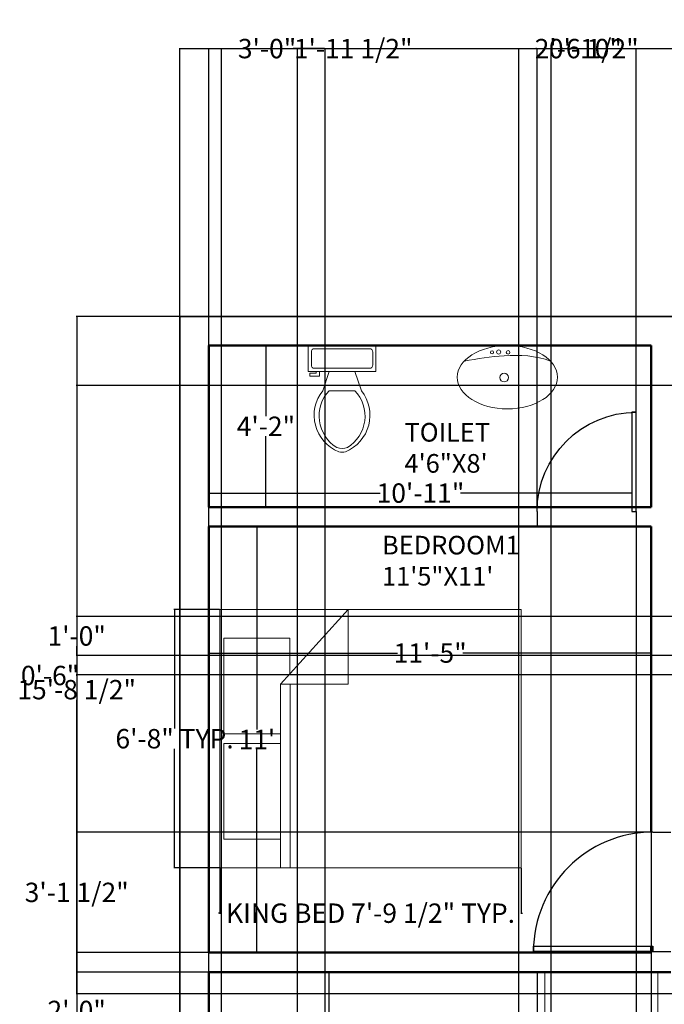
# Model space of a CAD drawing. Units: inches. Extents: x -56 to 545, y -536 to 185.
# Tile 5 of 7: x -56 to 144, y -120 to 185. Entities that reach past the tile are written whole.
import ezdxf

# ---------------------------------------------------------------- set-up
doc = ezdxf.new("R2010")
doc.units = ezdxf.units.IN
doc.header["$MEASUREMENT"] = 0
for name, color, linetype, lineweight in [('A-ANNO-DIMS', 2, 'Continuous', 18), ('A-AREA-IDEN', 4, 'Continuous', 25), ('A-DOOR', 4, 'Continuous', 25), ('A-EQPM', 9, 'Continuous', 18), ('A-FLOR-CASE', 8, 'Continuous', 25), ('A-FLOR-FIXT', 8, 'Continuous', 18), ('A-FURN', 8, 'Continuous', 18), ('A-WALL', 7, 'Continuous', 50), ('C-PROP', 7, 'Continuous', 35)]:
    doc.layers.add(name, color=color, linetype=linetype, lineweight=lineweight)
doc.styles.get("Standard").update_dxf_attribs({"font": 'arial.ttf'})
doc.dimstyles.get("Standard").update_dxf_attribs({"dimtxt": 6, "dimasz": 0.18, "dimexe": 0.18, "dimexo": 0.0625, "dimgap": 0.09, "dimtad": 0, "dimtih": 1, "dimtoh": 1, "dimdec": 0, "dimzin": 0, "dimdsep": 46, "dimlunit": 3, "dimtxsty": 'Standard', "dimcen": 0.09, "dimclrd": 3, "dimclre": 3, "dimclrt": 3, "dimadec": 0, "dimazin": 0, "dimtfac": 1, "dimtdec": 0, "dimtofl": 0, "dimtmove": 0, "dimatfit": 3, "dimfxl": 1, "dimtolj": 1, "dimtzin": 0, "dimarcsym": 0})

# ---------------------------------------------------------------- blocks, each defined once
blk = doc.blocks.new('CAMAKING')
for points in [[(0.8635, 0), (-0.8635, 0)], [(-0.8635, -2.0147), (-0.8635, 0)], [(0.8635, 0), (0.8635, -2.0147)], [(-0.6723, -0.4077), (-0.6723, -0.0281)], [(-0.6723, -0.0281), (-0.0328, -0.0281)], [(-0.0328, -0.0281), (-0.0328, -0.4077)], [(0.6716, -0.027), (0.0319, -0.027)], [(0.0319, -0.027), (0.0319, -0.4077)], [(0.6716, -0.4686), (0.6716, -0.027)], [(0.3645, -0.4056), (-0.8635, -0.4056)], [(0.8635, -0.857), (0.3645, -0.4056)], [(0.3645, -0.4702), (0.3645, -0.4056)], [(-0.8635, -0.4702), (0.3645, -0.4702)], [(0.3645, -0.4702), (0.3645, -0.857)], [(0.4362, -0.4686), (0.6716, -0.4686)], [(0.3645, -0.857), (0.8635, -0.857)], [(0.8635, -2.0147), (-0.8635, -2.0147)]]:
    blk.add_lwpolyline(points)
blk = doc.blocks.new('*U5')
for p, q in [((9.5, -6), (9.5, -2)), ((-10, -8.5), (-8, -8.5)), ((-10, -9.5), (-10, -8.5)), ((-8, -8.5), (-8, -8)), ((-7, -8), (-7, -9.5)), ((-4, -8), (-6, -14)), ((4, -8), (6, -14)), ((-7, -9.5), (-10, -9.5)), ((4, -14), (-4, -14))]:
    blk.add_line(p, q)
blk.add_lwpolyline([(10.5, -8), (10.5, 0), (-10.5, 0), (-10.5, -8)], close=True)
for points in [[(-9.5, -2), (-9.5, -6)], [(8.5, -1), (-8.5, -1)], [(-8.5, -7), (8.5, -7)]]:
    blk.add_lwpolyline(points)
for centre, radius, start, end in [((-8.62, -1.88), 0.884, 81.8699, 188.1301), ((8.62, -1.88), 0.884, 351.8699, 98.1301), ((-8.62, -6.12), 0.884, 171.8699, 278.1301), ((8.62, -6.12), 0.884, 261.8699, 8.1301), ((3.52, -21.58), 12.17, 141.4691, 247.9714), ((4.2, -21.82), 11.33, 136.3677, 238.9468), ((-3.52, -21.58), 12.17, 292.0284, 38.5307), ((-4.2, -21.82), 11.33, 301.053, 43.6321), ((0, -27.88), 4, 245.7318, 294.2682), ((0, -29), 4, 254.8605, 285.1395)]:
    blk.add_arc(centre, radius, start, end)
blk = doc.blocks.new('*U7')
for p, q in [((0, 0), (0, -6)), ((40, 0), (40, -6))]:
    blk.add_line(p, q)
blk.add_lwpolyline([(0, 0), (0, 40), (1.75, 40), (1.75, 0)], close=True)
blk.add_arc((0, 0), 40, 0, 90)
blk = doc.blocks.new('*D20')
at = {"layer": 'A-ANNO-DIMS', "color": 0, "lineweight": -2, "transparency": 16777216}
for p, q in [((96.89, -109.84), (40.02, -109.84)), ((40.2, -110.02), (40.2, -166.69)), ((40.2, -229.66), (40.2, -172.99)), ((96.89, -229.84), (40.02, -229.84))]:
    blk.add_line(p, q, dxfattribs=at)
at = {"layer": 'A-ANNO-DIMS', "color": 0, "transparency": 16777216}
for points in [[(40.17, -110.02), (40.23, -110.02), (40.2, -109.84)], [(40.17, -229.66), (40.23, -229.66), (40.2, -229.84)]]:
    blk.add_solid(points, dxfattribs=at)
at = {"layer": 'Defpoints', "color": 0, "transparency": 16777216}
for p in [(40.2, -109.84), (96.96, -109.84), (96.96, -229.84)]:
    blk.add_point(p, dxfattribs=at)
at = {"layer": 'A-ANNO-DIMS', "color": 0, "transparency": 16777216, "insert": (40.2, -169.84), "char_height": 6, "attachment_point": 5}
blk.add_mtext("\\A1;10'", dxfattribs=at)
blk = doc.blocks.new('*D22')
at = {"layer": 'A-ANNO-DIMS', "color": 0, "lineweight": -2, "transparency": 16777216}
for p, q in [((17.82, 28.16), (17.7, 28.16)), ((17.88, 27.98), (17.88, -34.74)), ((17.88, -103.66), (17.88, -40.94)), ((17.82, -103.84), (17.7, -103.84))]:
    blk.add_line(p, q, dxfattribs=at)
at = {"layer": 'A-ANNO-DIMS', "color": 0, "transparency": 16777216}
for points in [[(17.85, 27.98), (17.91, 27.98), (17.88, 28.16)], [(17.85, -103.66), (17.91, -103.66), (17.88, -103.84)]]:
    blk.add_solid(points, dxfattribs=at)
at = {"layer": 'Defpoints', "color": 0, "transparency": 16777216}
for p in [(17.88, 28.16), (17.88, 28.16), (17.88, -103.84)]:
    blk.add_point(p, dxfattribs=at)
at = {"layer": 'A-ANNO-DIMS', "color": 0, "transparency": 16777216, "insert": (17.88, -37.84), "char_height": 6, "attachment_point": 5}
blk.add_mtext("\\A1;11'", dxfattribs=at)
blk = doc.blocks.new('*D23')
at = {"layer": 'A-ANNO-DIMS', "color": 0, "lineweight": -2, "transparency": 16777216}
for p, q in [((3.03, 8), (3.03, -11.25)), ((140.03, 8), (140.03, -11.25)), ((3.21, -11.07), (61.42, -11.07)), ((139.85, -11.07), (81.65, -11.07))]:
    blk.add_line(p, q, dxfattribs=at)
at = {"layer": 'A-ANNO-DIMS', "color": 0, "transparency": 16777216}
for points in [[(3.21, -11.04), (3.21, -11.1), (3.03, -11.07)], [(139.85, -11.04), (139.85, -11.1), (140.03, -11.07)]]:
    blk.add_solid(points, dxfattribs=at)
at = {"layer": 'Defpoints', "color": 0, "transparency": 16777216}
for p in [(3.03, 8.06), (140.03, 8.06), (140.03, -11.07)]:
    blk.add_point(p, dxfattribs=at)
at = {"layer": 'A-ANNO-DIMS', "color": 0, "transparency": 16777216, "insert": (71.53, -11.07), "char_height": 6, "attachment_point": 5}
blk.add_mtext('\\A1;11\'-5"', dxfattribs=at)
blk = doc.blocks.new('*D24')
at = {"layer": 'A-ANNO-DIMS', "color": 0, "lineweight": -2, "transparency": 16777216}
for p, q in [((20.61, 84.16), (20.49, 84.16)), ((20.67, 83.98), (20.67, 62.26)), ((20.67, 34.34), (20.67, 56.06)), ((20.61, 34.16), (20.49, 34.16))]:
    blk.add_line(p, q, dxfattribs=at)
at = {"layer": 'A-ANNO-DIMS', "color": 0, "transparency": 16777216}
for points in [[(20.64, 83.98), (20.7, 83.98), (20.67, 84.16)], [(20.64, 34.34), (20.7, 34.34), (20.67, 34.16)]]:
    blk.add_solid(points, dxfattribs=at)
at = {"layer": 'Defpoints', "color": 0, "transparency": 16777216}
for p in [(20.67, 84.16), (20.67, 84.16), (20.67, 34.16)]:
    blk.add_point(p, dxfattribs=at)
at = {"layer": 'A-ANNO-DIMS', "color": 0, "transparency": 16777216, "insert": (20.67, 59.16), "char_height": 6, "attachment_point": 5}
blk.add_mtext('\\A1;4\'-2"', dxfattribs=at)
blk = doc.blocks.new('*D25')
at = {"layer": 'A-ANNO-DIMS', "color": 0, "lineweight": -2, "transparency": 16777216}
for p, q in [((3.03, 53.76), (3.03, 38.29)), ((134.04, 53.76), (134.04, 38.29)), ((3.21, 38.47), (56.09, 38.47)), ((133.86, 38.47), (80.98, 38.47))]:
    blk.add_line(p, q, dxfattribs=at)
at = {"layer": 'A-ANNO-DIMS', "color": 0, "transparency": 16777216}
for points in [[(3.21, 38.5), (3.21, 38.44), (3.03, 38.47)], [(133.86, 38.5), (133.86, 38.44), (134.04, 38.47)]]:
    blk.add_solid(points, dxfattribs=at)
at = {"layer": 'Defpoints', "color": 0, "transparency": 16777216}
for p in [(3.03, 53.82), (134.04, 53.82), (134.04, 38.47)]:
    blk.add_point(p, dxfattribs=at)
at = {"layer": 'A-ANNO-DIMS', "color": 0, "transparency": 16777216, "insert": (68.54, 38.47), "char_height": 6, "attachment_point": 5}
blk.add_mtext('\\A1;10\'-11"', dxfattribs=at)
blk = doc.blocks.new('LAV-OVAL')
for centre, radius in [((-4.76, 7.71), 0.472), ((-2.71, 7.81), 0.633), ((0.21, 7.71), 0.565), ((-1.02, -0.12), 1.35)]:
    blk.add_circle(centre, radius)
blk.add_ellipse((0, 0), major_axis=(-15.53, 0), ratio=0.631418)
blk.add_open_spline([(-13.36, 5), (-9.28, 5.7), (-0.46, 7.23), (8.86, 6.68), (13.36, 5)], degree=3, knots=[0, 0, 0, 0, 12.471835, 26.932887, 26.932887, 26.932887, 26.932887])
blk = doc.blocks.new('*D37')
at = {"layer": 'A-ANNO-DIMS', "color": 3, "lineweight": -2, "transparency": 16777216}
for p, q in [((6.38, -77.67), (6.38, -91.8)), ((99.76, -77.67), (99.76, -91.8)), ((6.2, -91.62), (6.02, -91.62)), ((99.94, -91.62), (100.12, -91.62))]:
    blk.add_line(p, q, dxfattribs=at)
at = {"layer": 'A-ANNO-DIMS', "color": 3, "transparency": 16777216}
for points in [[(6.2, -91.59), (6.2, -91.65), (6.38, -91.62)], [(99.94, -91.59), (99.94, -91.65), (99.76, -91.62)]]:
    blk.add_solid(points, dxfattribs=at)
at = {"layer": 'Defpoints', "color": 0, "transparency": 16777216}
for p in [(6.38, -77.61), (99.76, -77.61), (6.38, -91.62)]:
    blk.add_point(p, dxfattribs=at)
at = {"layer": 'A-ANNO-DIMS', "color": 3, "transparency": 16777216, "insert": (53.07, -91.62), "char_height": 6, "attachment_point": 5}
blk.add_mtext('\\A1;KING BED 7\'-9 1/2" TYP.', dxfattribs=at)
blk = doc.blocks.new('*D38')
at = {"layer": 'A-ANNO-DIMS', "color": 3, "lineweight": -2, "transparency": 16777216}
for p, q in [((6.32, 2.43), (-7.8, 2.43)), ((-7.62, 2.25), (-7.62, -34.43)), ((-7.62, -77.43), (-7.62, -40.74)), ((6.32, -77.61), (-7.8, -77.61))]:
    blk.add_line(p, q, dxfattribs=at)
at = {"layer": 'A-ANNO-DIMS', "color": 3, "transparency": 16777216}
for points in [[(-7.65, 2.25), (-7.59, 2.25), (-7.62, 2.43)], [(-7.65, -77.43), (-7.59, -77.43), (-7.62, -77.61)]]:
    blk.add_solid(points, dxfattribs=at)
at = {"layer": 'Defpoints', "color": 0, "transparency": 16777216}
for p in [(-7.62, 2.43), (6.38, 2.43), (6.38, -77.61)]:
    blk.add_point(p, dxfattribs=at)
at = {"layer": 'A-ANNO-DIMS', "color": 3, "transparency": 16777216, "insert": (-7.62, -37.59), "char_height": 6, "attachment_point": 5}
blk.add_mtext('\\A1;6\'-8" TYP.', dxfattribs=at)
blk = doc.blocks.new('*D52')
at = {"layer": 'A-ANNO-DIMS', "color": 3, "lineweight": -2, "transparency": 16777216}
for p, q in [((-6.03, 93.16), (-38.11, 93.16)), ((-37.93, 92.98), (-37.93, -197.69)), ((-37.93, -494.66), (-37.93, -203.99)), ((-6.03, -494.84), (-38.11, -494.84))]:
    blk.add_line(p, q, dxfattribs=at)
at = {"layer": 'A-ANNO-DIMS', "color": 3, "transparency": 16777216}
for points in [[(-37.96, 92.98), (-37.9, 92.98), (-37.93, 93.16)], [(-37.96, -494.66), (-37.9, -494.66), (-37.93, -494.84)]]:
    blk.add_solid(points, dxfattribs=at)
at = {"layer": 'Defpoints', "color": 0, "transparency": 16777216}
for p in [(-5.97, 93.16), (-37.93, -494.84), (-5.97, -494.84)]:
    blk.add_point(p, dxfattribs=at)
at = {"layer": 'A-ANNO-DIMS', "color": 3, "transparency": 16777216, "insert": (-37.93, -200.84), "char_height": 6, "attachment_point": 5}
blk.add_mtext('\\A1;49\'-0"', dxfattribs=at)
blk = doc.blocks.new('*D55')
at = {"layer": 'A-ANNO-DIMS', "color": 3, "lineweight": -2, "transparency": 16777216}
for p, q in [((290.97, -11.84), (-38.11, -11.84)), ((-37.93, -12.02), (-37.93, -17.66)), ((290.97, -17.84), (-38.11, -17.84)), ((-37.93, -18.02), (-38.11, -18.02)), ((-37.93, -17.84), (-37.93, -18.02))]:
    blk.add_line(p, q, dxfattribs=at)
at = {"layer": 'A-ANNO-DIMS', "color": 3, "transparency": 16777216}
for points in [[(-37.96, -12.02), (-37.9, -12.02), (-37.93, -11.84)], [(-37.96, -17.66), (-37.9, -17.66), (-37.93, -17.84)]]:
    blk.add_solid(points, dxfattribs=at)
at = {"layer": 'Defpoints', "color": 0, "transparency": 16777216}
for p in [(291.03, -11.84), (-37.93, -17.84), (291.03, -17.84)]:
    blk.add_point(p, dxfattribs=at)
at = {"layer": 'A-ANNO-DIMS', "color": 3, "transparency": 16777216, "insert": (-46.18, -18.02), "char_height": 6, "attachment_point": 5}
blk.add_mtext('\\A1;0\'-6"', dxfattribs=at)
blk = doc.blocks.new('*D56')
at = {"layer": 'A-ANNO-DIMS', "color": 3, "lineweight": -2, "transparency": 16777216}
for p, q in [((3.03, -235.78), (3.03, 176.3)), ((3.21, 176.12), (12.97, 176.12)), ((38.85, 176.12), (29.1, 176.12)), ((39.03, -235.78), (39.03, 176.3))]:
    blk.add_line(p, q, dxfattribs=at)
at = {"layer": 'A-ANNO-DIMS', "color": 3, "transparency": 16777216}
for points in [[(3.21, 176.15), (3.21, 176.09), (3.03, 176.12)], [(38.85, 176.15), (38.85, 176.09), (39.03, 176.12)]]:
    blk.add_solid(points, dxfattribs=at)
at = {"layer": 'Defpoints', "color": 0, "transparency": 16777216}
for p in [(39.03, 176.12), (3.03, -235.84), (39.03, -235.84)]:
    blk.add_point(p, dxfattribs=at)
at = {"layer": 'A-ANNO-DIMS', "color": 3, "transparency": 16777216, "insert": (21.03, 176.12), "char_height": 6, "attachment_point": 5}
blk.add_mtext('\\A1;3\'-0"', dxfattribs=at)
blk = doc.blocks.new('*D58')
at = {"layer": 'A-ANNO-DIMS', "color": 3, "lineweight": -2, "transparency": 16777216}
for p, q in [((99.03, -300.78), (99.03, 176.3)), ((99.21, 176.12), (108.85, 176.12)), ((109.03, -300.78), (109.03, 176.3)), ((109.03, 176.12), (109.21, 176.12))]:
    blk.add_line(p, q, dxfattribs=at)
at = {"layer": 'A-ANNO-DIMS', "color": 3, "transparency": 16777216}
for points in [[(99.21, 176.15), (99.21, 176.09), (99.03, 176.12)], [(108.85, 176.15), (108.85, 176.09), (109.03, 176.12)]]:
    blk.add_solid(points, dxfattribs=at)
at = {"layer": 'Defpoints', "color": 0, "transparency": 16777216}
for p in [(109.03, 176.12), (99.03, -300.84), (109.03, -300.84)]:
    blk.add_point(p, dxfattribs=at)
at = {"layer": 'A-ANNO-DIMS', "color": 3, "transparency": 16777216, "insert": (119.61, 176.12), "char_height": 6, "attachment_point": 5}
blk.add_mtext('\\A1;0\'-10"', dxfattribs=at)
blk = doc.blocks.new('*D67')
at = {"layer": 'A-ANNO-DIMS', "color": 3, "lineweight": -2, "transparency": 16777216}
for p, q in [((139.97, -66.51), (-38.11, -66.51)), ((-37.93, -66.69), (-37.93, -81.98)), ((-37.93, -103.66), (-37.93, -88.37)), ((139.97, -103.84), (-38.11, -103.84))]:
    blk.add_line(p, q, dxfattribs=at)
at = {"layer": 'A-ANNO-DIMS', "color": 3, "transparency": 16777216}
for points in [[(-37.96, -66.69), (-37.9, -66.69), (-37.93, -66.51)], [(-37.96, -103.66), (-37.9, -103.66), (-37.93, -103.84)]]:
    blk.add_solid(points, dxfattribs=at)
at = {"layer": 'Defpoints', "color": 0, "transparency": 16777216}
for p in [(140.03, -66.51), (-37.93, -103.84), (140.03, -103.84)]:
    blk.add_point(p, dxfattribs=at)
at = {"layer": 'A-ANNO-DIMS', "color": 3, "transparency": 16777216, "insert": (-37.93, -85.18), "char_height": 6, "attachment_point": 5}
blk.add_mtext('\\A1;3\'-1 1/2"', dxfattribs=at)
blk = doc.blocks.new('*D70')
at = {"layer": 'A-ANNO-DIMS', "color": 3, "lineweight": -2, "transparency": 16777216}
for p, q in [((421.61, 71.8), (-38.11, 71.8)), ((-37.93, 71.62), (-37.93, -19.2)), ((-37.93, -116.42), (-37.93, -25.59)), ((388.85, -116.6), (-38.11, -116.6))]:
    blk.add_line(p, q, dxfattribs=at)
at = {"layer": 'A-ANNO-DIMS', "color": 3, "transparency": 16777216}
for points in [[(-37.96, 71.62), (-37.9, 71.62), (-37.93, 71.8)], [(-37.96, -116.42), (-37.9, -116.42), (-37.93, -116.6)]]:
    blk.add_solid(points, dxfattribs=at)
at = {"layer": 'Defpoints', "color": 0, "transparency": 16777216}
for p in [(421.67, 71.8), (-37.93, -116.6), (388.91, -116.6)]:
    blk.add_point(p, dxfattribs=at)
at = {"layer": 'A-ANNO-DIMS', "color": 3, "transparency": 16777216, "insert": (-37.93, -22.4), "char_height": 6, "attachment_point": 5}
blk.add_mtext('\\A1;15\'-8 1/2"', dxfattribs=at)
blk = doc.blocks.new('*D72')
at = {"layer": 'A-ANNO-DIMS', "color": 3, "lineweight": -2, "transparency": 16777216}
for p, q in [((289.58, 0.27), (-38.11, 0.27)), ((-37.93, 0.09), (-37.93, -2.63)), ((-37.93, -11.66), (-37.93, -8.94)), ((290.97, -11.84), (-38.11, -11.84))]:
    blk.add_line(p, q, dxfattribs=at)
at = {"layer": 'A-ANNO-DIMS', "color": 3, "transparency": 16777216}
for points in [[(-37.96, 0.09), (-37.9, 0.09), (-37.93, 0.27)], [(-37.96, -11.66), (-37.9, -11.66), (-37.93, -11.84)]]:
    blk.add_solid(points, dxfattribs=at)
at = {"layer": 'Defpoints', "color": 0, "transparency": 16777216}
for p in [(289.64, 0.27), (-37.93, -11.84), (291.03, -11.84)]:
    blk.add_point(p, dxfattribs=at)
at = {"layer": 'A-ANNO-DIMS', "color": 3, "transparency": 16777216, "insert": (-37.93, -5.78), "char_height": 6, "attachment_point": 5}
blk.add_mtext('\\A1;1\'-0"', dxfattribs=at)
blk = doc.blocks.new('*D73')
at = {"layer": 'A-ANNO-DIMS', "color": 3, "lineweight": -2, "transparency": 16777216}
for p, q in [((135.38, 28.1), (135.38, -526.99)), ((140.03, 28.1), (140.03, -526.99)), ((135.56, -526.81), (139.85, -526.81)), ((140.03, -526.81), (140.21, -526.81))]:
    blk.add_line(p, q, dxfattribs=at)
at = {"layer": 'A-ANNO-DIMS', "color": 3, "transparency": 16777216}
for points in [[(135.56, -526.78), (135.56, -526.84), (135.38, -526.81)], [(139.85, -526.78), (139.85, -526.84), (140.03, -526.81)]]:
    blk.add_solid(points, dxfattribs=at)
at = {"layer": 'Defpoints', "color": 0, "transparency": 16777216}
for p in [(135.38, 28.16), (140.03, 28.16), (140.03, -526.81)]:
    blk.add_point(p, dxfattribs=at)
at = {"layer": 'A-ANNO-DIMS', "color": 3, "transparency": 16777216, "insert": (155.27, -526.81), "char_height": 6, "attachment_point": 5}
blk.add_mtext('\\A1;0\'-4 1/2"', dxfattribs=at)
blk = doc.blocks.new('*D74')
at = {"layer": 'A-ANNO-DIMS', "color": 3, "lineweight": -2, "transparency": 16777216}
for p, q in [((104.48, 176.12), (104.3, 176.12)), ((104.66, 32.83), (104.66, 176.3)), ((135.38, 32.83), (135.38, 176.3)), ((135.56, 176.12), (135.74, 176.12))]:
    blk.add_line(p, q, dxfattribs=at)
at = {"layer": 'A-ANNO-DIMS', "color": 3, "transparency": 16777216}
for points in [[(104.48, 176.15), (104.48, 176.09), (104.66, 176.12)], [(135.56, 176.15), (135.56, 176.09), (135.38, 176.12)]]:
    blk.add_solid(points, dxfattribs=at)
at = {"layer": 'Defpoints', "color": 0, "transparency": 16777216}
for p in [(135.38, 176.12), (104.66, 32.77), (135.38, 32.77)]:
    blk.add_point(p, dxfattribs=at)
at = {"layer": 'A-ANNO-DIMS', "color": 3, "transparency": 16777216, "insert": (120.02, 176.12), "char_height": 6, "attachment_point": 5}
blk.add_mtext('\\A1;2\'-6 1/2"', dxfattribs=at)
blk = doc.blocks.new('*D76')
at = {"layer": 'A-ANNO-DIMS', "color": 3, "lineweight": -2, "transparency": 16777216}
for p, q in [((2.97, -109.84), (-38.11, -109.84)), ((-37.93, -110.02), (-37.93, -118.6)), ((-37.93, -133.48), (-37.93, -124.91)), ((33.44, -133.66), (-38.11, -133.66))]:
    blk.add_line(p, q, dxfattribs=at)
at = {"layer": 'A-ANNO-DIMS', "color": 3, "transparency": 16777216}
for points in [[(-37.96, -110.02), (-37.9, -110.02), (-37.93, -109.84)], [(-37.96, -133.48), (-37.9, -133.48), (-37.93, -133.66)]]:
    blk.add_solid(points, dxfattribs=at)
at = {"layer": 'Defpoints', "color": 0, "transparency": 16777216}
for p in [(3.03, -109.84), (-37.93, -133.66), (33.5, -133.66)]:
    blk.add_point(p, dxfattribs=at)
at = {"layer": 'A-ANNO-DIMS', "color": 3, "transparency": 16777216, "insert": (-37.93, -121.75), "char_height": 6, "attachment_point": 5}
blk.add_mtext('\\A1;2\'-0"', dxfattribs=at)
blk = doc.blocks.new('*D78')
at = {"layer": 'A-ANNO-DIMS', "color": 3, "lineweight": -2, "transparency": 16777216}
for p, q in [((6.93, -149.29), (6.93, 176.3)), ((7.11, 176.12), (30.24, 176.12)), ((30.42, -149.29), (30.42, 176.3)), ((30.42, 176.12), (30.6, 176.12))]:
    blk.add_line(p, q, dxfattribs=at)
at = {"layer": 'A-ANNO-DIMS', "color": 3, "transparency": 16777216}
for points in [[(7.11, 176.15), (7.11, 176.09), (6.93, 176.12)], [(30.24, 176.15), (30.24, 176.09), (30.42, 176.12)]]:
    blk.add_solid(points, dxfattribs=at)
at = {"layer": 'Defpoints', "color": 0, "transparency": 16777216}
for p in [(30.42, 176.12), (6.93, -149.35), (30.42, -149.35)]:
    blk.add_point(p, dxfattribs=at)
at = {"layer": 'A-ANNO-DIMS', "color": 3, "transparency": 16777216, "insert": (47.7, 176.12), "char_height": 6, "attachment_point": 5}
blk.add_mtext('\\A1;1\'-11 1/2"', dxfattribs=at)
blk = doc.blocks.new('*D90')
at = {"layer": 'A-ANNO-DIMS', "color": 3, "lineweight": -2, "transparency": 16777216}
for p, q in [((-5.97, 93.22), (-5.97, 176.3)), ((-5.79, 176.12), (163.64, 176.12)), ((353.85, 176.12), (184.43, 176.12)), ((354.03, 84.22), (354.03, 176.3))]:
    blk.add_line(p, q, dxfattribs=at)
at = {"layer": 'A-ANNO-DIMS', "color": 3, "transparency": 16777216}
for points in [[(-5.79, 176.15), (-5.79, 176.09), (-5.97, 176.12)], [(353.85, 176.15), (353.85, 176.09), (354.03, 176.12)]]:
    blk.add_solid(points, dxfattribs=at)
at = {"layer": 'Defpoints', "color": 0, "transparency": 16777216}
for p in [(354.03, 176.12), (-5.97, 93.16), (354.03, 84.16)]:
    blk.add_point(p, dxfattribs=at)
at = {"layer": 'A-ANNO-DIMS', "color": 3, "transparency": 16777216, "insert": (174.03, 176.12), "char_height": 6, "attachment_point": 5}
blk.add_mtext('\\A1;30\'-0"', dxfattribs=at)

msp = doc.modelspace()

# ---------------------------------------------------------------- linework, layer by layer
at = {"layer": 'A-EQPM'}
for p, q in [((107.02, -133.66), (107.02, -109.84)), ((142.07, -109.84), (142.07, -133.66))]:
    msp.add_line(p, q, dxfattribs=at)
at = {"layer": 'A-FLOR-CASE'}
msp.add_line((104.78, -133.66), (104.78, -109.84), dxfattribs=at)
at = {"layer": 'A-WALL'}
for p, q in [((3.03, 84.16), (140.03, 84.16)), ((3.03, 84.16), (3.03, 34.16)), ((140.03, 84.16), (140.03, 34.16)), ((3.03, 34.16), (140.03, 34.16)), ((3.03, 28.16), (140.03, 28.16)), ((3.03, 28.16), (3.03, -103.84)), ((140.03, 28.16), (140.03, -66.51)), ((140.03, -101.86), (140.03, -103.84)), ((3.03, -103.84), (140.03, -103.84)), ((3.03, -109.84), (122.03, -109.84)), ((3.03, -109.84), (3.03, -229.84)), ((122.03, -109.84), (146.03, -109.84))]:
    msp.add_line(p, q, dxfattribs=at)
at = {"layer": 'C-PROP'}
for q in [(-5.97, -494.84), (498.03, 93.16)]:
    msp.add_line((-5.97, 93.16), q, dxfattribs=at)

# ---------------------------------------------------------------- block references
at = {"layer": 'A-DOOR', "xscale": -0.7680778388986921, "yscale": 0.7680778388986921, "zscale": 0.7680778388986921}
msp.add_blockref('*U7', (135.38, 32.77), dxfattribs=at)
at = {"layer": 'A-DOOR', "xscale": 0.924222506201659, "yscale": 0.924222506201659, "zscale": 0.924222506201659, "rotation": 90}
msp.add_blockref('*U7', (140.49, -103.48), dxfattribs=at)
at = {"layer": 'A-FLOR-FIXT'}
for name, p in [('*U5', (44.25, 84.16)), ('LAV-OVAL', (95.46, 74.35))]:
    msp.add_blockref(name, p, dxfattribs=at)
at = {"layer": 'A-FURN', "xscale": 46.34928316146463, "yscale": 46.34928316146463, "zscale": 46.34928316146463, "rotation": 90}
msp.add_blockref('CAMAKING', (6.38, -37.59), dxfattribs=at)

# ---------------------------------------------------------------- texts
at = {"layer": 'A-AREA-IDEN', "char_height": 5.772, "attachment_point": 1}
for s, insert in [('{TOILET\\P4\'6"X8\'}', (63.59, 60.18)), ('{BEDROOM1\\P11\'5"X11\'}', (56.62, 25.24))]:
    msp.add_mtext_dynamic_manual_height_columns(s, width=1091.0728, gutter_width=28.86, heights=[0], dxfattribs=dict(at, insert=insert))

# ---------------------------------------------------------------- dimensions: what is measured, and where the dimension line sits
at = {"layer": 'A-ANNO-DIMS'}
for base, p1, p2, override, picture, middle in [((30.42, 176.12), (6.93, -149.35), (30.42, -149.35), {"dimdec": 1, "dimlfac": 1, "dimrnd": 0, "dimzin": 1, "dimdsep": 46, "dimlunit": 4, "dimfrac": 2}, '*D78', (47.7, 176.12)), ((135.38, 176.12), (104.66, 32.77), (135.38, 32.77), {"dimdec": 1, "dimlfac": 1, "dimrnd": 0, "dimzin": 1, "dimdsep": 46, "dimlunit": 4, "dimfrac": 2}, '*D74', (120.02, 176.12)), ((354.03, 176.12), (-5.97, 93.16), (354.03, 84.16), {"dimdec": 1, "dimlfac": 1, "dimrnd": 0, "dimzin": 1, "dimdsep": 46, "dimlunit": 4, "dimfrac": 2}, '*D90', (174.03, 176.12)), ((39.03, 176.12), (3.03, -235.84), (39.03, -235.84), {"dimdec": 1, "dimlfac": 1, "dimrnd": 0, "dimzin": 1, "dimdsep": 46, "dimlunit": 4, "dimfrac": 2}, '*D56', (21.03, 176.12)), ((109.03, 176.12), (99.03, -300.84), (109.03, -300.84), {"dimdec": 1, "dimlfac": 1, "dimrnd": 0, "dimzin": 1, "dimdsep": 46, "dimlunit": 4, "dimfrac": 2}, '*D58', (119.61, 176.12)), ((134.04, 38.47), (3.03, 53.82), (134.04, 53.82), {"dimclrd": 0, "dimclre": 0, "dimclrt": 0}, '*D25', (68.54, 38.47)), ((140.0343, -526.8056), (135.3838, 28.1594), (140.0343, 28.1594), {"dimdec": 1, "dimlfac": 1, "dimrnd": 0, "dimzin": 1, "dimdsep": 46, "dimlunit": 4, "dimfrac": 2}, '*D73', (155.2695, -526.8056)), ((140.03, -11.07), (3.03, 8.06), (140.03, 8.06), {"dimclrd": 0, "dimclre": 0, "dimclrt": 0}, '*D23', (71.53, -11.07))]:
    dim = msp.add_linear_dim(base=base, p1=p1, p2=p2, dimstyle='Standard', override=override, dxfattribs=at)
    dim.commit()
    dim.dimension.update_dxf_attribs({"geometry": picture, "text_midpoint": middle})
for base, p1, p2, override, picture, middle in [((-37.93, -494.84), (-5.97, 93.16), (-5.97, -494.84), {"dimdec": 1, "dimlfac": 1, "dimrnd": 0, "dimzin": 1, "dimdsep": 46, "dimlunit": 4, "dimfrac": 2}, '*D52', (-37.93, -200.84)), ((20.67, 84.16), (20.67, 34.16), (20.67, 84.16), {"dimclrd": 0, "dimclre": 0, "dimclrt": 0}, '*D24', (20.67, 59.16)), ((-37.93, -116.6), (421.67, 71.8), (388.91, -116.6), {"dimdec": 1, "dimlfac": 1, "dimrnd": 0, "dimzin": 1, "dimdsep": 46, "dimlunit": 4, "dimfrac": 2}, '*D70', (-37.93, -22.4)), ((17.88, 28.16), (17.88, -103.84), (17.88, 28.16), {"dimclrd": 0, "dimclre": 0, "dimclrt": 0}, '*D22', (17.88, -37.84)), ((-37.93, -11.84), (289.64, 0.27), (291.03, -11.84), {"dimdec": 1, "dimlfac": 1, "dimrnd": 0, "dimzin": 1, "dimdsep": 46, "dimlunit": 4, "dimfrac": 2}, '*D72', (-37.93, -5.78)), ((-37.93, -17.84), (291.03, -11.84), (291.03, -17.84), {"dimdec": 1, "dimlfac": 1, "dimrnd": 0, "dimzin": 1, "dimdsep": 46, "dimlunit": 4, "dimfrac": 2}, '*D55', (-46.18, -18.02)), ((-37.93, -103.84), (140.03, -66.51), (140.03, -103.84), {"dimdec": 1, "dimlfac": 1, "dimrnd": 0, "dimzin": 1, "dimdsep": 46, "dimlunit": 4, "dimfrac": 2}, '*D67', (-37.93, -85.18)), ((-37.93, -133.66), (3.03, -109.84), (33.5, -133.66), {"dimdec": 1, "dimlfac": 1, "dimrnd": 0, "dimzin": 1, "dimdsep": 46, "dimlunit": 4, "dimfrac": 2}, '*D76', (-37.93, -121.75)), ((40.2, -109.84), (96.96, -229.84), (96.96, -109.84), {"dimclrd": 0, "dimclre": 0, "dimclrt": 0}, '*D20', (40.2, -169.84))]:
    dim = msp.add_linear_dim(base=base, p1=p1, p2=p2, angle=90, dimstyle='Standard', override=override, dxfattribs=at)
    dim.commit()
    dim.dimension.update_dxf_attribs({"geometry": picture, "text_midpoint": middle})
for base, p1, p2, angle, text, picture, middle in [((-7.62, 2.43), (6.38, -77.61), (6.38, 2.43), 90, '<> TYP.', '*D38', (-7.62, -37.59)), ((6.38, -91.62), (99.76, -77.61), (6.38, -77.61), 180, 'KING BED <> TYP.', '*D37', (53.07, -91.62))]:
    dim = msp.add_linear_dim(base=base, p1=p1, p2=p2, angle=angle, text=text, dimstyle='Standard', override={"dimdec": 1, "dimlfac": 1, "dimrnd": 0, "dimzin": 1, "dimdsep": 46, "dimlunit": 4, "dimfrac": 2}, dxfattribs=at)
    dim.commit()
    dim.dimension.update_dxf_attribs({"geometry": picture, "text_midpoint": middle})

doc.saveas('drawing.dxf')
